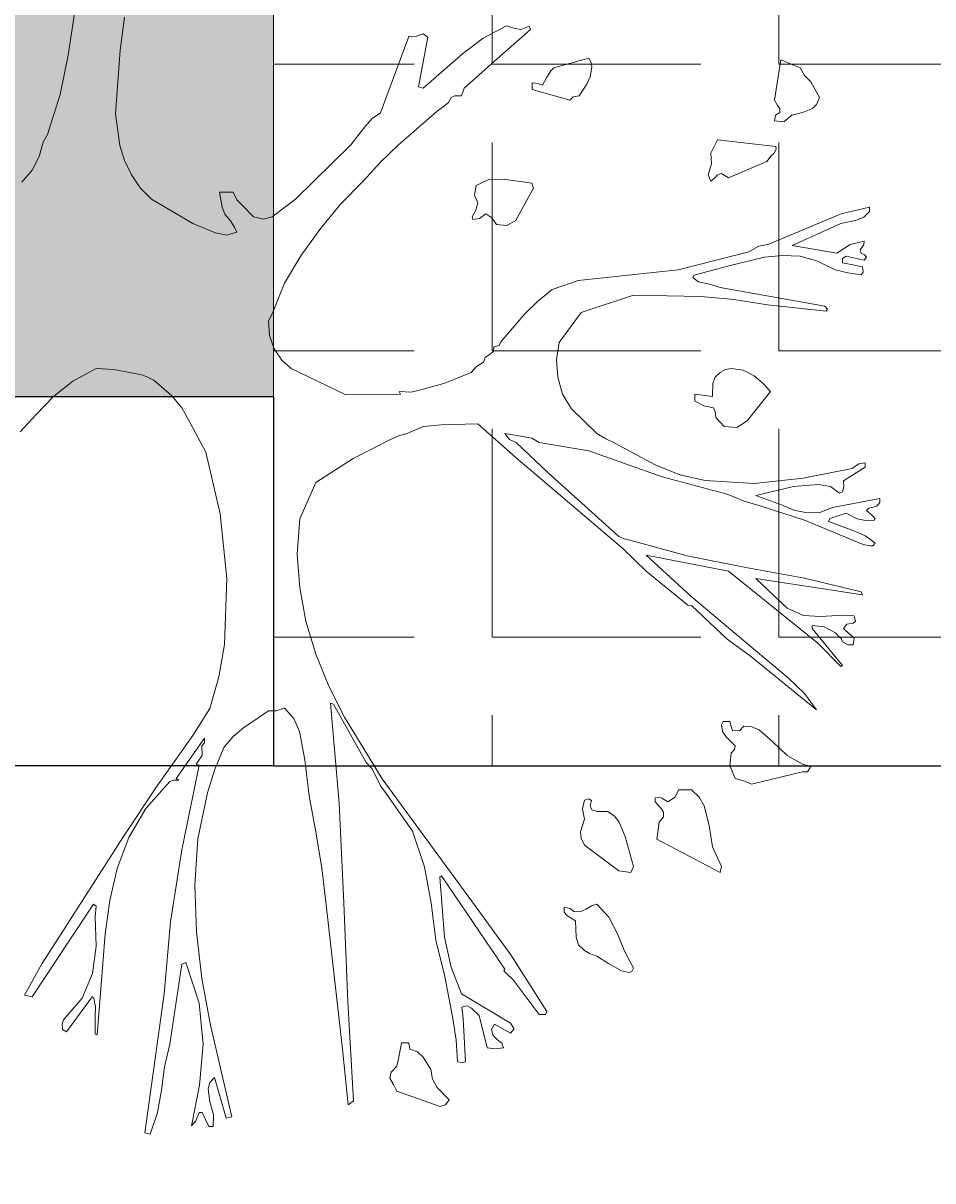
# Model space of a CAD drawing. Units: inches. Extents: x 84 to 1044, y -280 to 906.
# Tile 7 of 105: x 498 to 521, y -132 to -104. Entities that reach past the tile are written whole.
import ezdxf

# ---------------------------------------------------------------- set-up
doc = ezdxf.new("R2010")
doc.units = ezdxf.units.IN
for name, color, linetype, lineweight in [('A-ANNO-DIMS', 2, 'Continuous', 18), ('C-PROP', 7, 'Continuous', 25), ('L-HRDS', 32, 'Continuous', 18), ('L-PLNT', 114, 'Continuous', 15)]:
    doc.layers.add(name, color=color, linetype=linetype, lineweight=lineweight)
doc.layers.add('L-HRDS-PATT', color=23, linetype='Continuous', lineweight=9, true_color=0xc2877b)
doc.layers.add('L-PLNT-PATT', color=9, linetype='Continuous', lineweight=9, true_color=0xafd9aa)
doc.styles.get("Standard").update_dxf_attribs({"font": 'arial.ttf'})
doc.dimstyles.get("Standard").update_dxf_attribs({"dimtxt": 0.18, "dimasz": 0.18, "dimexe": 0.18, "dimexo": 0.0625, "dimgap": 0.09, "dimtad": 0, "dimtih": 1, "dimtoh": 1, "dimdec": 4, "dimzin": 0, "dimdsep": 46, "dimtxsty": 'Standard', "dimcen": 0.09, "dimadec": 0, "dimazin": 0, "dimtfac": 1, "dimtdec": 4, "dimtofl": 0, "dimtmove": 0, "dimatfit": 3, "dimfxl": 1, "dimtolj": 1, "dimtzin": 0, "dimarcsym": 0})

# ---------------------------------------------------------------- blocks, each defined once
blk = doc.blocks.new('A$C37E508DF')
for p, q in [((0.7911, 1.1436), (0.8027, 1.0677)), ((0.7512, 1.0728), (0.7469, 1.1054)), ((0.3456, 1.093), (0.3469, 1.0964)), ((0.3842, 1.0591), (0.3456, 1.093)), ((0.3469, 1.0964), (0.355, 1.093)), ((0.355, 1.093), (0.3619, 1.0943)), ((0.3619, 1.0943), (0.3692, 1.0968)), ((0.3692, 1.0968), (0.3923, 1.0844)), ((0.4472, 1.0857), (0.4515, 1.0887)), ((0.4515, 1.0887), (0.4584, 1.0865)), ((0.3923, 1.0844), (0.4129, 1.069)), ((0.4562, 1.0364), (0.4472, 1.0857)), ((0.4584, 1.0865), (0.4657, 1.0861)), ((0.4657, 1.0861), (0.4939, 1.0107)), ((0.4129, 1.069), (0.4515, 1.0351)), ((0.7538, 1.0415), (0.7512, 1.0728)), ((0.8027, 1.0677), (0.8108, 1.0287)), ((0.0746, 1.0475), (0.0789, 1.0552)), ((0.0789, 1.0552), (0.0978, 1.063)), ((0.0978, 1.063), (0.1042, 1.0231)), ((0.2847, 1.0565), (0.2856, 1.0604)), ((0.2851, 1.054), (0.2847, 1.0565)), ((0.2864, 1.0463), (0.2851, 1.054)), ((0.2856, 1.0604), (0.2877, 1.0647)), ((0.2877, 1.0647), (0.3224, 1.0552)), ((0.3224, 1.0552), (0.3255, 1.0522)), ((0.4112, 1.0351), (0.3842, 1.0591)), ((0.0682, 1.0415), (0.0746, 1.0475)), ((0.2899, 1.039), (0.2864, 1.0463)), ((0.3255, 1.0522), (0.3293, 1.0458)), ((0.3293, 1.0458), (0.3336, 1.0381)), ((0.0596, 1.0257), (0.0682, 1.0415)), ((0.2972, 1.0274), (0.2899, 1.039)), ((0.3439, 1.0338), (0.3066, 1.0231)), ((0.3336, 1.0381), (0.3383, 1.0398)), ((0.3383, 1.0398), (0.3439, 1.0402)), ((0.3439, 1.0402), (0.3439, 1.0338)), ((0.4138, 1.0274), (0.4112, 1.0351)), ((0.4515, 1.0351), (0.4562, 1.0364)), ((0.7559, 1.0098), (0.7538, 1.0415)), ((0.0626, 1.0188), (0.0596, 1.0257)), ((0.1042, 1.0231), (0.1012, 1.018)), ((0.3032, 1.0265), (0.2972, 1.0274)), ((0.3066, 1.0231), (0.3032, 1.0265)), ((0.4202, 1.0274), (0.4138, 1.0274)), ((0.4241, 1.0257), (0.4202, 1.0274)), ((0.4267, 1.0209), (0.4241, 1.0257)), ((0.4305, 1.0175), (0.4267, 1.0209)), ((0.8108, 1.0287), (0.8233, 0.9892)), ((0.0665, 1.0149), (0.0626, 1.0188)), ((0.0763, 1.0111), (0.0665, 1.0149)), ((0.087, 1.0085), (0.0763, 1.0111)), ((0.0948, 1.0016), (0.087, 1.0085)), ((0.1012, 1.018), (0.099, 1.0149)), ((0.099, 1.0149), (0.099, 1.0111)), ((0.099, 1.0111), (0.1033, 1.0085)), ((0.1033, 1.0085), (0.1042, 1.0029)), ((0.4378, 1.0124), (0.4305, 1.0175)), ((0.476, 0.9789), (0.4378, 1.0124)), ((0.4939, 1.0107), (0.5021, 1.0051)), ((0.7516, 0.9785), (0.7559, 1.0098)), ((0.1042, 1.0029), (0.0948, 1.0016)), ((0.5021, 1.0051), (0.5094, 0.9969)), ((0.5094, 0.9969), (0.5231, 0.9789)), ((0.8233, 0.9892), (0.8275, 0.9815)), ((0.1025, 0.9751), (0.1029, 0.9772)), ((0.1046, 0.9708), (0.1025, 0.9751)), ((0.1029, 0.9772), (0.1604, 0.9841)), ((0.1604, 0.9841), (0.1672, 0.9708)), ((0.4939, 0.9618), (0.476, 0.9789)), ((0.5231, 0.9789), (0.578, 0.9253)), ((0.7469, 0.9635), (0.7516, 0.9785)), ((0.8275, 0.9815), (0.8314, 0.9673)), ((0.1076, 0.9682), (0.1046, 0.9708)), ((0.1119, 0.9626), (0.1076, 0.9682)), ((0.1496, 0.9463), (0.1119, 0.9626)), ((0.1672, 0.9708), (0.1664, 0.9601)), ((0.7401, 0.9493), (0.7469, 0.9635)), ((0.8314, 0.9673), (0.8383, 0.954)), ((0.1664, 0.9601), (0.1698, 0.9493)), ((0.5111, 0.9429), (0.4939, 0.9618)), ((0.8383, 0.954), (0.8486, 0.942)), ((0.1565, 0.9506), (0.1496, 0.9463)), ((0.1604, 0.9493), (0.1565, 0.9506)), ((0.1629, 0.9468), (0.1604, 0.9493)), ((0.1672, 0.9429), (0.1629, 0.9468)), ((0.1698, 0.9493), (0.1672, 0.9429)), ((0.3426, 0.936), (0.3443, 0.9412)), ((0.3443, 0.9412), (0.3722, 0.9451)), ((0.3722, 0.9451), (0.3868, 0.9446)), ((0.3868, 0.9446), (0.3992, 0.9386)), ((0.5334, 0.9202), (0.5111, 0.9429)), ((0.7315, 0.9365), (0.7401, 0.9493)), ((0.3602, 0.9039), (0.3426, 0.936)), ((0.4009, 0.9292), (0.3975, 0.9215)), ((0.3992, 0.9386), (0.4009, 0.9292)), ((0.6359, 0.9245), (0.6397, 0.9322)), ((0.6397, 0.9322), (0.653, 0.9322)), ((0.653, 0.9322), (0.6505, 0.9172)), ((0.7203, 0.9253), (0.7315, 0.9365)), ((0.0103, 0.9129), (0.0103, 0.9172)), ((0.0103, 0.9172), (0.0382, 0.9107)), ((0.3975, 0.9215), (0.3996, 0.9142)), ((0.554, 0.8953), (0.5334, 0.9202)), ((0.578, 0.9253), (0.6011, 0.9077)), ((0.6196, 0.9077), (0.6303, 0.9189)), ((0.6303, 0.9189), (0.6359, 0.9245)), ((0.6505, 0.9172), (0.6479, 0.9103)), ((0.6796, 0.9013), (0.7203, 0.9253)), ((0.0159, 0.9073), (0.0103, 0.9129)), ((0.0232, 0.9043), (0.0159, 0.9073)), ((0.0382, 0.9107), (0.1098, 0.8807)), ((0.3838, 0.9069), (0.379, 0.9)), ((0.3898, 0.9107), (0.3838, 0.9069)), ((0.3958, 0.906), (0.3898, 0.9107)), ((0.4026, 0.9052), (0.3958, 0.906)), ((0.3996, 0.9142), (0.4031, 0.9077)), ((0.4031, 0.9077), (0.4026, 0.9052)), ((0.6011, 0.9077), (0.6097, 0.9056)), ((0.6097, 0.9056), (0.6196, 0.9077)), ((0.6479, 0.9103), (0.6423, 0.9039)), ((0.0386, 0.9013), (0.0232, 0.9043)), ((0.0866, 0.8794), (0.0386, 0.9013)), ((0.3692, 0.8992), (0.3602, 0.9039)), ((0.379, 0.9), (0.3692, 0.8992)), ((0.5728, 0.8691), (0.554, 0.8953)), ((0.6384, 0.8974), (0.6359, 0.8927)), ((0.6423, 0.9039), (0.6384, 0.8974)), ((0.6569, 0.8919), (0.6796, 0.9013)), ((0.0159, 0.8803), (0.0154, 0.8837)), ((0.0154, 0.8837), (0.0292, 0.8803)), ((0.6359, 0.8927), (0.6457, 0.8897)), ((0.6457, 0.8897), (0.6569, 0.8919)), ((0.015, 0.87), (0.0184, 0.8717)), ((0.0176, 0.8777), (0.0159, 0.8803)), ((0.0193, 0.8752), (0.0176, 0.8777)), ((0.0184, 0.8717), (0.0193, 0.8752)), ((0.0292, 0.8803), (0.0424, 0.8717)), ((0.0424, 0.8717), (0.0866, 0.8794)), ((0.1098, 0.8807), (0.1196, 0.8786)), ((0.1196, 0.8786), (0.1295, 0.873)), ((0.1295, 0.873), (0.1994, 0.8554)), ((0.0133, 0.8679), (0.015, 0.87)), ((0.0154, 0.8649), (0.0133, 0.8679)), ((0.0334, 0.8687), (0.0154, 0.8649)), ((0.0171, 0.8584), (0.0266, 0.8602)), ((0.0266, 0.8602), (0.0369, 0.8623)), ((0.0369, 0.8666), (0.0334, 0.8687)), ((0.0369, 0.8623), (0.0369, 0.8666)), ((0.0617, 0.864), (0.0442, 0.8554)), ((0.0789, 0.8687), (0.0617, 0.864)), ((0.0965, 0.8696), (0.0789, 0.8687)), ((0.1141, 0.8679), (0.0965, 0.8696)), ((0.1492, 0.8593), (0.1141, 0.8679)), ((0.1835, 0.8499), (0.1492, 0.8593)), ((0.5887, 0.8421), (0.5728, 0.8691)), ((0.0163, 0.8529), (0.0171, 0.8584)), ((0.0184, 0.8503), (0.0163, 0.8529)), ((0.0317, 0.8524), (0.0184, 0.8503)), ((0.0442, 0.8554), (0.0317, 0.8524)), ((0.1848, 0.8477), (0.1835, 0.8499)), ((0.1994, 0.8554), (0.2984, 0.8447)), ((0.0545, 0.8194), (0.1578, 0.8378)), ((0.1578, 0.8378), (0.1698, 0.8413)), ((0.1698, 0.8413), (0.1792, 0.8434)), ((0.1792, 0.8434), (0.1848, 0.8477)), ((0.2984, 0.8447), (0.3242, 0.8357)), ((0.6007, 0.8125), (0.5887, 0.8421)), ((0.1441, 0.8258), (0.1111, 0.8207)), ((0.1771, 0.8288), (0.1441, 0.8258)), ((0.2436, 0.8301), (0.1771, 0.8288)), ((0.2954, 0.813), (0.2436, 0.8301)), ((0.3242, 0.8357), (0.3387, 0.8241)), ((0.0519, 0.8164), (0.0545, 0.8194)), ((0.0532, 0.8143), (0.0519, 0.8164)), ((0.1111, 0.8207), (0.0532, 0.8143)), ((0.3387, 0.8241), (0.3512, 0.8117)), ((0.3173, 0.7834), (0.2954, 0.813)), ((0.3512, 0.8117), (0.3748, 0.7842)), ((0.6046, 0.8048), (0.6007, 0.8125)), ((0.6037, 0.7903), (0.6046, 0.8048)), ((0.3199, 0.7662), (0.3173, 0.7834)), ((0.3748, 0.7842), (0.3765, 0.7804)), ((0.3765, 0.7804), (0.3816, 0.7791)), ((0.3816, 0.7791), (0.382, 0.7744)), ((0.599, 0.777), (0.6037, 0.7903)), ((0.382, 0.7744), (0.3859, 0.7714)), ((0.3859, 0.7714), (0.3902, 0.7684)), ((0.3902, 0.7684), (0.3919, 0.7641)), ((0.5913, 0.7658), (0.599, 0.777)), ((0.1351, 0.7559), (0.1471, 0.7577)), ((0.1471, 0.7577), (0.1527, 0.7568)), ((0.1527, 0.7568), (0.1578, 0.7538)), ((0.3186, 0.7491), (0.3199, 0.7662)), ((0.3919, 0.7641), (0.3988, 0.7598)), ((0.3988, 0.7598), (0.4043, 0.7538)), ((0.5287, 0.7319), (0.5823, 0.7577)), ((0.5823, 0.7577), (0.5913, 0.7658)), ((0.7577, 0.7568), (0.7401, 0.7534)), ((0.7752, 0.7577), (0.7577, 0.7568)), ((0.798, 0.7452), (0.7752, 0.7577)), ((0.1153, 0.7427), (0.1244, 0.7504)), ((0.1244, 0.7504), (0.1351, 0.7559)), ((0.1578, 0.7538), (0.1629, 0.7491)), ((0.1629, 0.7491), (0.1651, 0.7431)), ((0.3139, 0.7324), (0.3186, 0.7491)), ((0.4043, 0.7538), (0.4301, 0.7431)), ((0.7182, 0.7461), (0.7002, 0.7307)), ((0.7285, 0.7512), (0.7182, 0.7461)), ((0.7401, 0.7534), (0.7285, 0.7512)), ((0.8173, 0.7298), (0.798, 0.7452)), ((0.1081, 0.7349), (0.1153, 0.7427)), ((0.1312, 0.7058), (0.1081, 0.7349)), ((0.1651, 0.7431), (0.1655, 0.7298)), ((0.4301, 0.7431), (0.4515, 0.7371)), ((0.4515, 0.7371), (0.4635, 0.7341)), ((0.4635, 0.7341), (0.4755, 0.7349)), ((0.4755, 0.7349), (0.4742, 0.7324)), ((0.1655, 0.7298), (0.1831, 0.7324)), ((0.1831, 0.7255), (0.1741, 0.7208)), ((0.1831, 0.7324), (0.1831, 0.7255)), ((0.3049, 0.7178), (0.3139, 0.7324)), ((0.4742, 0.7324), (0.5287, 0.7319)), ((0.7002, 0.7307), (0.6903, 0.7186)), ((0.8344, 0.7122), (0.8173, 0.7298)), ((0.1629, 0.7152), (0.1621, 0.7092)), ((0.1646, 0.7186), (0.1629, 0.7152)), ((0.1741, 0.7208), (0.1646, 0.7186)), ((0.28, 0.6933), (0.3049, 0.7178)), ((0.6903, 0.7186), (0.6818, 0.7032)), ((0.8503, 0.6951), (0.8344, 0.7122)), ((0.1415, 0.6994), (0.1312, 0.7058)), ((0.1539, 0.7002), (0.1415, 0.6994)), ((0.1621, 0.7092), (0.1539, 0.7002)), ((0.3975, 0.7028), (0.3598, 0.6693)), ((0.4339, 0.7019), (0.3975, 0.7028)), ((0.4515, 0.7002), (0.4339, 0.7019)), ((0.4674, 0.6933), (0.4515, 0.7002)), ((0.6818, 0.7032), (0.6667, 0.6749)), ((0.262, 0.6839), (0.271, 0.6882)), ((0.271, 0.6882), (0.28, 0.6933)), ((0.3443, 0.6886), (0.337, 0.6843)), ((0.3533, 0.6903), (0.3443, 0.6886)), ((0.3709, 0.6933), (0.3533, 0.6903)), ((0.3662, 0.6873), (0.3709, 0.6933)), ((0.476, 0.6912), (0.4674, 0.6933)), ((0.4832, 0.6878), (0.476, 0.6912)), ((0.521, 0.6685), (0.4832, 0.6878)), ((0.2877, 0.6762), (0.2152, 0.6505)), ((0.2221, 0.6625), (0.262, 0.6839)), ((0.337, 0.6843), (0.2877, 0.6762)), ((0.328, 0.6543), (0.3598, 0.6843)), ((0.3598, 0.6843), (0.3662, 0.6873)), ((0.3598, 0.6693), (0.2543, 0.5797)), ((0.5578, 0.6449), (0.521, 0.6685)), ((0.6667, 0.6749), (0.6526, 0.614)), ((0.0146, 0.6599), (0.0146, 0.6642)), ((0.0146, 0.6642), (0.0206, 0.6633)), ((0.036, 0.6466), (0.0146, 0.6599)), ((0.0206, 0.6633), (0.0274, 0.6586)), ((0.0274, 0.6586), (0.0759, 0.6492)), ((0.1977, 0.6526), (0.2221, 0.6625)), ((0.2581, 0.5913), (0.328, 0.6543)), ((0.0356, 0.6406), (0.036, 0.6466)), ((0.0609, 0.6428), (0.0489, 0.641)), ((0.0853, 0.641), (0.0609, 0.6428)), ((0.0759, 0.6492), (0.1244, 0.644)), ((0.1244, 0.644), (0.1728, 0.647)), ((0.2152, 0.6505), (0.1509, 0.6333)), ((0.1728, 0.647), (0.1977, 0.6526)), ((0.5737, 0.6089), (0.5578, 0.6449)), ((0.0369, 0.6355), (0.0356, 0.6406)), ((0.0399, 0.6342), (0.0369, 0.6355)), ((0.0489, 0.641), (0.0399, 0.6342)), ((0.1226, 0.632), (0.0853, 0.641)), ((0.0973, 0.6226), (0.1226, 0.632)), ((0.1509, 0.6333), (0.1342, 0.6265)), ((0, 0.629), (0.0467, 0.62)), ((0, 0.6252), (0, 0.629)), ((0.003, 0.6213), (0, 0.6252)), ((0.0069, 0.6204), (0.003, 0.6213)), ((0.0107, 0.6196), (0.0069, 0.6204)), ((0.0133, 0.617), (0.0107, 0.6196)), ((0.0467, 0.62), (0.0592, 0.6153)), ((0.1175, 0.6213), (0.0746, 0.6076)), ((0.0849, 0.6175), (0.0973, 0.6226)), ((0.1342, 0.6265), (0.1175, 0.6213)), ((0.0047, 0.6093), (0.0086, 0.6132)), ((0.0056, 0.6076), (0.0047, 0.6093)), ((0.0141, 0.6072), (0.0056, 0.6076)), ((0.0086, 0.6132), (0.0133, 0.617)), ((0.0223, 0.6089), (0.0141, 0.6072)), ((0.0746, 0.6076), (0.0163, 0.5836)), ((0.0334, 0.6145), (0.0223, 0.6089)), ((0.0416, 0.6119), (0.0334, 0.6145)), ((0.0493, 0.6093), (0.0416, 0.6119)), ((0.0506, 0.6063), (0.0493, 0.6093)), ((0.0592, 0.6153), (0.072, 0.6149)), ((0.072, 0.6149), (0.0849, 0.6175)), ((0.5763, 0.5741), (0.5737, 0.6089)), ((0.6526, 0.614), (0.6457, 0.5497)), ((0.0141, 0.5921), (0.0257, 0.5969)), ((0.0257, 0.5969), (0.0506, 0.6063)), ((0.0047, 0.5849), (0.0141, 0.5921)), ((0.0069, 0.5823), (0.0047, 0.5849)), ((0.1904, 0.5724), (0.2474, 0.5879)), ((0.2474, 0.5879), (0.253, 0.5892)), ((0.253, 0.5892), (0.2581, 0.5913)), ((0.0099, 0.5823), (0.0069, 0.5823)), ((0.0163, 0.5836), (0.0099, 0.5823)), ((0.2311, 0.5729), (0.1496, 0.557)), ((0.1869, 0.5325), (0.2311, 0.5729)), ((0.2543, 0.5797), (0.2311, 0.557)), ((0.5737, 0.5407), (0.5763, 0.5741)), ((0.1325, 0.5608), (0.1904, 0.5724)), ((0.0184, 0.5368), (0.0746, 0.5501)), ((0.1496, 0.557), (0.0613, 0.4858)), ((0.0746, 0.5501), (0.1325, 0.5608)), ((0.2311, 0.557), (0.1899, 0.5235)), ((0.1226, 0.5497), (0.0171, 0.5338)), ((0.0917, 0.5205), (0.1226, 0.5497)), ((0.5677, 0.5077), (0.5737, 0.5407)), ((0.6457, 0.5497), (0.6483, 0.4845)), ((0.0171, 0.5338), (0.0184, 0.5368)), ((0.1269, 0.482), (0.1869, 0.5325)), ((0.0755, 0.5133), (0.0917, 0.5205)), ((0.1861, 0.5231), (0.1509, 0.4897)), ((0.1899, 0.5235), (0.1861, 0.5231)), ((0.024, 0.5072), (0.0253, 0.5128)), ((0.0262, 0.5055), (0.024, 0.5072)), ((0.0253, 0.5128), (0.042, 0.5133)), ((0.0326, 0.5047), (0.0262, 0.5055)), ((0.036, 0.5004), (0.0326, 0.5047)), ((0.042, 0.5133), (0.0587, 0.5124)), ((0.0587, 0.5124), (0.0755, 0.5133)), ((0.5578, 0.4751), (0.5677, 0.5077)), ((0.0253, 0.491), (0.03, 0.4948)), ((0.03, 0.4948), (0.036, 0.5004)), ((0.0369, 0.4639), (0.0669, 0.5004)), ((0.0437, 0.4961), (0.0403, 0.4922)), ((0.0549, 0.5021), (0.0437, 0.4961)), ((0.0669, 0.5034), (0.0549, 0.5021)), ((0.0669, 0.5004), (0.0669, 0.5034)), ((0.0262, 0.4841), (0.0253, 0.491)), ((0.0317, 0.4841), (0.0262, 0.4841)), ((0.0369, 0.4871), (0.0317, 0.4841)), ((0.0382, 0.4905), (0.0369, 0.4871)), ((0.0403, 0.4922), (0.0382, 0.4905)), ((0.0613, 0.4858), (0.0386, 0.4627)), ((0.0905, 0.4515), (0.1269, 0.482)), ((0.1509, 0.4897), (0.1282, 0.4734)), ((0.6483, 0.4845), (0.6539, 0.4524)), ((0.1282, 0.4734), (0.0626, 0.4198)), ((0.545, 0.4434), (0.5578, 0.4751)), ((0.0386, 0.4627), (0.0369, 0.4639)), ((0.0746, 0.4361), (0.0905, 0.4515)), ((0.6539, 0.4524), (0.6625, 0.4211)), ((0.0626, 0.4198), (0.0746, 0.4361)), ((0.5295, 0.4125), (0.545, 0.4434)), ((0.5403, 0.4254), (0.5081, 0.3679)), ((0.5347, 0.3276), (0.5433, 0.4266)), ((0.5433, 0.4266), (0.5403, 0.4254)), ((0.4922, 0.3516), (0.5295, 0.4125)), ((0.5887, 0.4215), (0.5797, 0.4112)), ((0.5969, 0.4189), (0.5887, 0.4215)), ((0.6046, 0.4189), (0.5969, 0.4189)), ((0.6295, 0.4022), (0.6046, 0.4189)), ((0.6625, 0.4211), (0.6796, 0.3945)), ((0.1192, 0.4001), (0.1265, 0.4031)), ((0.1265, 0.4031), (0.1346, 0.4039)), ((0.1346, 0.4039), (0.1389, 0.3992)), ((0.1458, 0.3996), (0.1471, 0.4035)), ((0.1471, 0.4035), (0.1484, 0.4082)), ((0.1484, 0.4082), (0.1548, 0.4082)), ((0.1548, 0.4082), (0.1565, 0.4052)), ((0.1565, 0.4052), (0.1556, 0.3983)), ((0.5797, 0.4112), (0.5741, 0.3983)), ((0.6397, 0.3936), (0.6295, 0.4022)), ((0.1055, 0.388), (0.1192, 0.4001)), ((0.1389, 0.3992), (0.1458, 0.3996)), ((0.1518, 0.3932), (0.1432, 0.3842)), ((0.1556, 0.3983), (0.1518, 0.3932)), ((0.5741, 0.3983), (0.5686, 0.3705)), ((0.6487, 0.3825), (0.6397, 0.3936)), ((0.6959, 0.352), (0.668, 0.3919)), ((0.668, 0.3919), (0.668, 0.3872)), ((0.6796, 0.3945), (0.7148, 0.3447)), ((0.0917, 0.3748), (0.1055, 0.388)), ((0.1432, 0.3842), (0.1436, 0.3808)), ((0.1436, 0.3808), (0.1471, 0.3769)), ((0.6582, 0.3602), (0.6487, 0.3825)), ((0.668, 0.3872), (0.6706, 0.3842)), ((0.6706, 0.3842), (0.6702, 0.3748)), ((0.0763, 0.3662), (0.0917, 0.3748)), ((0.1471, 0.3769), (0.1484, 0.3649)), ((0.5081, 0.3679), (0.5025, 0.3619)), ((0.5686, 0.3705), (0.5643, 0.3349)), ((0.6702, 0.3748), (0.6762, 0.3662)), ((0.069, 0.364), (0.0763, 0.3662)), ((0.069, 0.3627), (0.069, 0.364)), ((0.0716, 0.3585), (0.069, 0.3627)), ((0.0763, 0.3585), (0.0716, 0.3585)), ((0.1269, 0.3464), (0.0763, 0.3585)), ((0.1484, 0.3649), (0.1432, 0.352)), ((0.5025, 0.3619), (0.4982, 0.3537)), ((0.665, 0.3379), (0.6582, 0.3602)), ((0.6762, 0.3662), (0.6732, 0.3653)), ((0.6732, 0.3653), (0.6903, 0.2813)), ((0.1355, 0.3499), (0.1269, 0.3464)), ((0.1432, 0.352), (0.1355, 0.3499)), ((0.4065, 0.2345), (0.4922, 0.3516)), ((0.4939, 0.3447), (0.4884, 0.337)), ((0.4982, 0.3537), (0.4939, 0.3447)), ((0.6933, 0.3503), (0.6959, 0.352)), ((0.6985, 0.3503), (0.6933, 0.3503)), ((0.7023, 0.349), (0.6985, 0.3503)), ((0.7259, 0.3224), (0.7023, 0.349)), ((0.7148, 0.3447), (0.7487, 0.2937)), ((0.1737, 0.325), (0.1788, 0.3336)), ((0.1788, 0.3336), (0.1861, 0.3409)), ((0.1861, 0.3409), (0.199, 0.3409)), ((0.199, 0.3409), (0.2024, 0.3336)), ((0.2024, 0.3336), (0.2097, 0.3289)), ((0.2097, 0.3289), (0.2148, 0.3323)), ((0.2148, 0.3323), (0.2182, 0.3336)), ((0.2182, 0.3336), (0.2221, 0.3327)), ((0.2221, 0.3327), (0.2221, 0.3289)), ((0.4884, 0.337), (0.4622, 0.2997)), ((0.5643, 0.3349), (0.5578, 0.2993)), ((0.6745, 0.2924), (0.665, 0.3379)), ((0.1689, 0.3053), (0.1737, 0.325)), ((0.2161, 0.3224), (0.214, 0.3186)), ((0.2221, 0.3289), (0.2161, 0.3224)), ((0.2796, 0.3194), (0.2847, 0.3211)), ((0.2847, 0.3211), (0.2864, 0.325)), ((0.2851, 0.3302), (0.2877, 0.3319)), ((0.2864, 0.325), (0.2851, 0.3302)), ((0.2877, 0.3319), (0.292, 0.3306)), ((0.292, 0.3306), (0.2941, 0.322)), ((0.2941, 0.322), (0.292, 0.3117)), ((0.53, 0.229), (0.5347, 0.3276)), ((0.7427, 0.2937), (0.7259, 0.3224)), ((0.214, 0.3186), (0.214, 0.3139)), ((0.214, 0.3139), (0.2182, 0.3087)), ((0.2577, 0.3087), (0.2624, 0.3147)), ((0.2624, 0.3147), (0.2689, 0.3194)), ((0.2689, 0.3194), (0.2796, 0.3194)), ((0.292, 0.3117), (0.2959, 0.2993)), ((0.1655, 0.2843), (0.1689, 0.3053)), ((0.2182, 0.3087), (0.2204, 0.292)), ((0.2517, 0.2946), (0.2577, 0.3087)), ((0.2959, 0.2993), (0.2954, 0.2928)), ((0.4622, 0.2997), (0.4502, 0.2645)), ((0.5578, 0.2993), (0.5518, 0.2633)), ((0.2204, 0.292), (0.1578, 0.259)), ((0.2436, 0.265), (0.2517, 0.2946)), ((0.2954, 0.2928), (0.292, 0.286)), ((0.6775, 0.2465), (0.6745, 0.2924)), ((0.7542, 0.2628), (0.7427, 0.2937)), ((0.7487, 0.2937), (0.8151, 0.1899)), ((0.1565, 0.265), (0.1655, 0.2843)), ((0.292, 0.286), (0.2581, 0.2607)), ((0.6903, 0.2813), (0.7015, 0.2101)), ((0.1578, 0.259), (0.1565, 0.265)), ((0.2461, 0.259), (0.2436, 0.265)), ((0.4502, 0.2645), (0.4438, 0.2285)), ((0.2581, 0.2607), (0.2461, 0.259)), ((0.4335, 0.2556), (0.3709, 0.1634)), ((0.4305, 0.1951), (0.4352, 0.2543)), ((0.4352, 0.2543), (0.4335, 0.2556)), ((0.5518, 0.2633), (0.5475, 0.2268)), ((0.7615, 0.2311), (0.7542, 0.2628)), ((0.6758, 0.2002), (0.6775, 0.2465)), ((0.3649, 0.1775), (0.4065, 0.2345)), ((0.7662, 0.1981), (0.7615, 0.2311)), ((0.268, 0.2148), (0.28, 0.2277)), ((0.28, 0.2277), (0.2851, 0.226)), ((0.2851, 0.226), (0.2903, 0.2225)), ((0.2903, 0.2225), (0.2963, 0.22)), ((0.2963, 0.22), (0.3027, 0.2204)), ((0.3027, 0.2204), (0.3061, 0.2234)), ((0.3061, 0.2234), (0.3122, 0.2247)), ((0.3122, 0.22), (0.3096, 0.2165)), ((0.3122, 0.2247), (0.3122, 0.22)), ((0.4438, 0.2285), (0.4391, 0.1921)), ((0.5261, 0.1308), (0.53, 0.229)), ((0.5475, 0.2268), (0.5313, 0.084)), ((0.7778, 0.2277), (0.7752, 0.2255)), ((0.7752, 0.2255), (0.7761, 0.2152)), ((0.8018, 0.1912), (0.7778, 0.2277)), ((0.2594, 0.1981), (0.268, 0.2148)), ((0.301, 0.211), (0.3002, 0.1951)), ((0.3096, 0.2165), (0.301, 0.211)), ((0.7015, 0.2101), (0.7079, 0.1389)), ((0.7761, 0.2152), (0.7752, 0.1861)), ((0.2521, 0.1805), (0.2594, 0.1981)), ((0.3002, 0.1951), (0.298, 0.1874)), ((0.4241, 0.1651), (0.4305, 0.1951)), ((0.6706, 0.1539), (0.6758, 0.2002)), ((0.7688, 0.1646), (0.7662, 0.1981)), ((0.298, 0.1874), (0.292, 0.1818)), ((0.4391, 0.1921), (0.4301, 0.1561)), ((0.7752, 0.1861), (0.7787, 0.1591)), ((0.8383, 0.1359), (0.8018, 0.1912)), ((0.8151, 0.1899), (0.8288, 0.1685)), ((0.2436, 0.1642), (0.2521, 0.1805)), ((0.28, 0.1762), (0.2684, 0.1689)), ((0.2873, 0.1788), (0.28, 0.1762)), ((0.292, 0.1818), (0.2873, 0.1788)), ((0.3293, 0.1213), (0.3649, 0.1775)), ((0.2448, 0.1616), (0.2436, 0.1642)), ((0.2478, 0.1599), (0.2448, 0.1616)), ((0.2508, 0.1608), (0.2478, 0.1599)), ((0.2556, 0.1616), (0.2508, 0.1608)), ((0.2684, 0.1689), (0.2556, 0.1616)), ((0.3718, 0.1616), (0.3692, 0.1591)), ((0.3709, 0.1634), (0.3718, 0.1616)), ((0.4138, 0.1389), (0.4241, 0.1651)), ((0.6865, 0.1698), (0.6732, 0.1295)), ((0.6903, 0.1681), (0.6865, 0.1698)), ((0.7023, 0.0892), (0.6903, 0.1681)), ((0.774, 0.0982), (0.7688, 0.1646)), ((0.8288, 0.1685), (0.846, 0.1376)), ((0.3628, 0.1526), (0.337, 0.1183)), ((0.3692, 0.1591), (0.3628, 0.1526)), ((0.4301, 0.1561), (0.4224, 0.1145)), ((0.662, 0.108), (0.6706, 0.1539)), ((0.7787, 0.1591), (0.789, 0.1346)), ((0.3653, 0.1098), (0.4138, 0.1389)), ((0.7079, 0.1389), (0.7268, 0.0013)), ((0.846, 0.1376), (0.8383, 0.1359)), ((0.4082, 0.1269), (0.4039, 0.1248)), ((0.4134, 0.1256), (0.4082, 0.1269)), ((0.5205, 0.033), (0.5261, 0.1308)), ((0.6732, 0.1295), (0.6693, 0.0892)), ((0.7774, 0.1346), (0.7757, 0.1261)), ((0.7757, 0.1261), (0.7761, 0.117)), ((0.7791, 0.1359), (0.7774, 0.1346)), ((0.8044, 0.1012), (0.7791, 0.1359)), ((0.789, 0.1346), (0.8074, 0.1132)), ((0.3306, 0.1183), (0.3293, 0.1213)), ((0.337, 0.1183), (0.3306, 0.1183)), ((0.3962, 0.1175), (0.3885, 0.0853)), ((0.4039, 0.1248), (0.3962, 0.1175)), ((0.4121, 0.1145), (0.4134, 0.1256)), ((0.7761, 0.117), (0.7761, 0.099)), ((0.3615, 0.1042), (0.3653, 0.1098)), ((0.3653, 0.0999), (0.3615, 0.1042)), ((0.3812, 0.1089), (0.3653, 0.0999)), ((0.3842, 0.1037), (0.3812, 0.1089)), ((0.3825, 0.0978), (0.3842, 0.1037)), ((0.4099, 0.0716), (0.4121, 0.1145)), ((0.4224, 0.1145), (0.4189, 0.093)), ((0.641, 0.0172), (0.662, 0.108)), ((0.8083, 0.1037), (0.8044, 0.1012)), ((0.8074, 0.1132), (0.8087, 0.1089)), ((0.8087, 0.1089), (0.8083, 0.1037)), ((0.3739, 0.09), (0.3782, 0.0935)), ((0.3782, 0.0935), (0.3825, 0.0978)), ((0.4189, 0.093), (0.4176, 0.072)), ((0.7761, 0.099), (0.774, 0.0982)), ((0.3722, 0.0853), (0.3739, 0.09)), ((0.3808, 0.0845), (0.3722, 0.0853)), ((0.3885, 0.0853), (0.3808, 0.0845)), ((0.4515, 0.0763), (0.4571, 0.0815)), ((0.4571, 0.0815), (0.4648, 0.084)), ((0.4648, 0.084), (0.4657, 0.0905)), ((0.4657, 0.0905), (0.473, 0.0905)), ((0.473, 0.0905), (0.476, 0.0746)), ((0.5313, 0.084), (0.5257, 0.0291)), ((0.6693, 0.0892), (0.6728, 0.0484)), ((0.7075, 0.0665), (0.7023, 0.0892)), ((0.4142, 0.0707), (0.4099, 0.0716)), ((0.4176, 0.072), (0.4142, 0.0707)), ((0.4442, 0.0639), (0.4515, 0.0763)), ((0.476, 0.0746), (0.4777, 0.0673)), ((0.4425, 0.0544), (0.4442, 0.0639)), ((0.4777, 0.0673), (0.4832, 0.0613)), ((0.4832, 0.0613), (0.4845, 0.0553)), ((0.7105, 0.0437), (0.7075, 0.0665)), ((0.4258, 0.0339), (0.4378, 0.0463)), ((0.4378, 0.0463), (0.4425, 0.0544)), ((0.4811, 0.0493), (0.4777, 0.0424)), ((0.4845, 0.0553), (0.4811, 0.0493)), ((0.6582, 0.0562), (0.6466, 0.0159)), ((0.6625, 0.051), (0.6582, 0.0562)), ((0.6642, 0.045), (0.6625, 0.051)), ((0.6728, 0.0484), (0.6809, 0.0082)), ((0.4777, 0.0424), (0.4348, 0.0274)), ((0.6625, 0.0321), (0.6642, 0.045)), ((0.7144, 0.0214), (0.7105, 0.0437)), ((0.4296, 0.0291), (0.4258, 0.0339)), ((0.4348, 0.0274), (0.4296, 0.0291)), ((0.5257, 0.0291), (0.5205, 0.033)), ((0.659, 0.0193), (0.6625, 0.0321)), ((0.6466, 0.0159), (0.641, 0.0172)), ((0.6595, 0.0077), (0.659, 0.0193)), ((0.6702, 0.0214), (0.6637, 0.0077)), ((0.6732, 0.0214), (0.6702, 0.0214)), ((0.6766, 0.0133), (0.6732, 0.0214)), ((0.6809, 0.0082), (0.6766, 0.0133)), ((0.7216, 0), (0.7144, 0.0214)), ((0.6637, 0.0077), (0.6595, 0.0077)), ((0.7268, 0.0013), (0.7216, 0))]:
    blk.add_line(p, q)
blk = doc.blocks.new('*D60')
at = {"layer": 'A-ANNO-DIMS', "color": 0, "lineweight": -2, "transparency": 16777216}
for p, q in [((134.179, -121.942), (134.179, -180.64)), ((992.074, -121.942), (992.074, -180.64)), ((134.359, -180.46), (562.733, -180.46)), ((991.894, -180.46), (563.521, -180.46))]:
    blk.add_line(p, q, dxfattribs=at)
at = {"layer": 'A-ANNO-DIMS', "color": 0, "transparency": 16777216}
for points in [[(134.359, -180.43), (134.359, -180.49), (134.179, -180.46)], [(991.894, -180.43), (991.894, -180.49), (992.074, -180.46)]]:
    blk.add_solid(points, dxfattribs=at)
at = {"layer": 'Defpoints', "color": 0, "transparency": 16777216}
for p in [(134.179, -121.88), (992.074, -121.88), (992.074, -180.46)]:
    blk.add_point(p, dxfattribs=at)
at = {"layer": 'A-ANNO-DIMS', "color": 0, "transparency": 16777216, "insert": (563.127, -180.46), "char_height": 0.18, "attachment_point": 5}
blk.add_mtext('\\A1;857.9', dxfattribs=at)

msp = doc.modelspace()

# ---------------------------------------------------------------- hatches: boundary and pattern name
at = {"layer": 'L-HRDS-PATT', "transparency": 33554567}
h = msp.add_hatch(dxfattribs=at)
h.set_pattern_fill('ANGLE', color=256)
h.set_pattern_definition([(0, (0, 0), (0, 6.985), [5.08, -1.905]), (90, (0, 0), (-6.985, 4e-16), [5.08, -1.905])])
h.paths.add_polyline_path([(650.074, 31.12), (504.574, 31.12), (504.574, -112.88), (504.574, -121.88), (624.574, -121.88), (624.574, -112.88), (650.074, -112.88)])
at = {"layer": 'L-PLNT-PATT', "transparency": 33554597}
h = msp.add_hatch(color=256, dxfattribs=at)
h.dxf.hatch_style = 1
h.paths.add_polyline_path([(504.574, -40.88), (455.074, -40.88), (455.074, -112.88), (504.574, -112.88)])

# ---------------------------------------------------------------- linework, layer by layer
at = {"layer": 'C-PROP'}
for p, q in [((504.574, -112.88), (504.574, -121.88)), ((504.574, -121.88), (624.574, -121.88))]:
    msp.add_line(p, q, dxfattribs=at)
for points in [[(504.574, -112.88), (455.074, -112.88)], [(504.574, -121.88), (455.074, -121.88)]]:
    msp.add_lwpolyline(points, dxfattribs=at)
at = {"layer": 'L-HRDS'}
msp.add_line((504.574, -112.88), (504.574, 31.12), dxfattribs=at)

# ---------------------------------------------------------------- block references
at = {"layer": 'L-PLNT', "xscale": -24.64361536662419, "yscale": 24.64361536662419, "zscale": 24.64361536662419}
msp.add_blockref('A$C37E508DF', (519.355, -130.86), dxfattribs=at)

# ---------------------------------------------------------------- dimensions: what is measured, and where the dimension line sits
at = {"layer": 'A-ANNO-DIMS'}
dim = msp.add_linear_dim(base=(992.074, -180.46), p1=(134.179, -121.88), p2=(992.074, -121.88), dimstyle='Standard', override={"dimdec": 1, "dimlfac": 1, "dimrnd": 0, "dimzin": 0, "dimdsep": 46, "dimlunit": 2}, dxfattribs=at)
dim.commit()
dim.dimension.update_dxf_attribs({"geometry": '*D60', "text_midpoint": (563.127, -180.46)})

doc.saveas('drawing.dxf')
